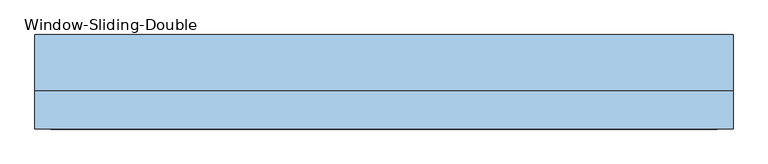
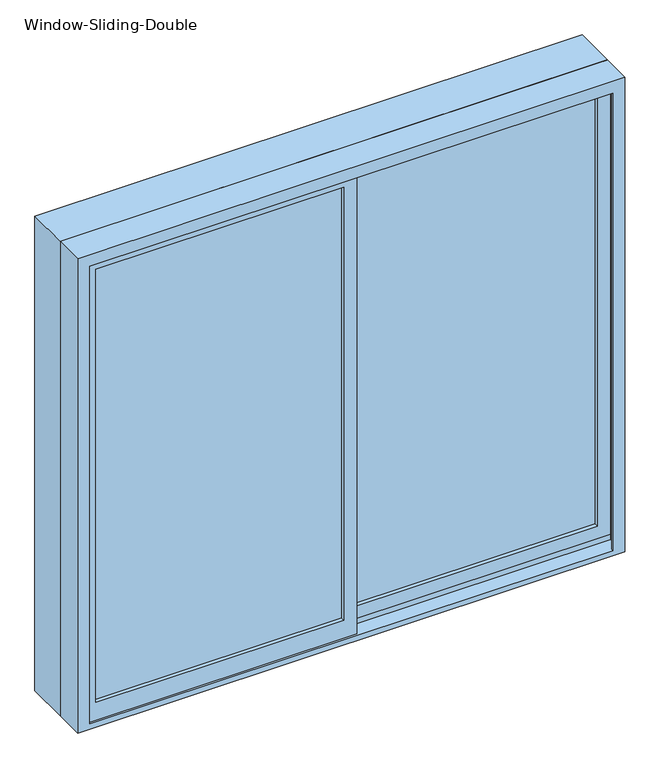
"""IFC4 building model written with IfcOpenShell, lengths in millimetres: window geometry, Window-Sliding-Double."""

from ifc_helpers import new_model, si_unit, frame, origin, place, context, project, spatial, polyline, outline, extrude, faceted_brep, source, transform, mapped, element, save


def window_sliding_double_c634d93e(model_context):
    return source(origin(), model_context, "Body", "SolidModel", [
        extrude(outline(polyline([(952.5, -22.225), (952.5, 895.35), (2571.75, 895.35), (2571.75, -22.225), (952.5, -22.225)]), holes=[polyline([(996.95, 850.9), (996.95, 22.225), (2527.3, 22.225), (2527.3, 850.9), (996.95, 850.9)])]), frame((0.0, -78.74, 0.0), z_axis=(0.0, 1.0, 0.0), x_axis=(0.0, 0.0, 1.0)), (0.0, 0.0, 1.0), 44.45),
        extrude(outline(polyline([(933.45, 22.225), (2571.75, 22.225), (2571.75, -895.35), (933.45, -895.35), (933.45, 22.225)]), holes=[polyline([(2527.3, -850.9), (2527.3, -22.225), (996.95, -22.225), (996.95, -850.9), (2527.3, -850.9)])]), frame((0.0, -123.19, 0.0), z_axis=(0.0, 1.0, 0.0), x_axis=(0.0, 0.0, 1.0)), (0.0, 0.0, 1.0), 44.45),
        extrude(outline(polyline([(-22.225, -110.49), (-850.9, -110.49), (-850.9, -104.14), (-22.225, -104.14), (-22.225, -110.49)])), frame((0.0, 0.0, 996.95), z_axis=(0.0, 0.0, 1.0), x_axis=(1.0, 0.0, 0.0)), (0.0, 0.0, 1.0), 1530.35),
        extrude(outline(polyline([(-22.225, -97.79), (-850.9, -97.79), (-850.9, -91.44), (-22.225, -91.44), (-22.225, -97.79)])), frame((0.0, 0.0, 996.95), z_axis=(0.0, 0.0, 1.0), x_axis=(1.0, 0.0, 0.0)), (0.0, 0.0, 1.0), 1530.35),
        extrude(outline(polyline([(850.9, -66.04), (22.225, -66.04), (22.225, -59.69), (850.9, -59.69), (850.9, -66.04)])), frame((0.0, 0.0, 996.95), z_axis=(0.0, 0.0, 1.0), x_axis=(1.0, 0.0, 0.0)), (0.0, 0.0, 1.0), 1530.35),
        extrude(outline(polyline([(850.9, -53.34), (22.225, -53.34), (22.225, -46.99), (850.9, -46.99), (850.9, -53.34)])), frame((0.0, 0.0, 996.95), z_axis=(0.0, 0.0, 1.0), x_axis=(1.0, 0.0, 0.0)), (0.0, 0.0, 1.0), 1530.35),
        extrude(outline(polyline([(2590.8, 914.4), (2590.8, -914.4), (914.4, -914.4), (914.4, 914.4), (2590.8, 914.4)]), holes=[polyline([(2571.75, -895.35), (2571.75, 895.35), (933.45, 895.35), (933.45, -895.35), (2571.75, -895.35)])]), frame((0.0, -27.94, 0.0), z_axis=(0.0, 1.0, 0.0), x_axis=(0.0, 0.0, 1.0)), (0.0, 0.0, 1.0), 146.05),
        faceted_brep([(-914.4, -27.94, 914.4), (914.4, -27.94, 914.4), (914.4, -129.54, 914.4), (-914.4, -129.54, 914.4), (-873.4778905, -129.54, 2549.8778905), (-873.4778905, -129.54, 933.45), (-873.4778905, -123.19, 933.45), (-873.4778905, -123.19, 2549.8778905), (-895.35, -123.19, 933.45), (-895.35, -123.19, 2571.75), (895.35, -123.19, 2571.75), (895.35, -123.19, 933.45), (873.4778905, -123.19, 933.45), (873.4778905, -123.19, 2549.8778905), (-895.35, -78.74, 933.45), (-895.35, -78.74, 952.5), (-895.35, -34.29, 952.5), (-895.35, -34.29, 933.45), (-895.35, -27.94, 933.45), (-895.35, -27.94, 2571.75), (-914.4, -27.94, 2590.8), (914.4, -27.94, 2590.8), (895.35, -27.94, 2571.75), (895.35, -27.94, 933.45), (-914.4, -129.54, 2590.8), (914.4, -129.54, 2590.8), (873.4778905, -129.54, 2549.8778905), (873.4778905, -129.54, 933.45), (895.35, -34.29, 933.45), (895.35, -34.29, 952.5), (895.35, -78.74, 952.5), (895.35, -78.74, 933.45)], [[[0, 1, 2, 3]], [[4, 5, 6, 7]], [[7, 6, 8, 9, 10, 11, 12, 13]], [[9, 8, 14, 15, 16, 17, 18, 19]], [[0, 20, 21, 1], [22, 19, 18, 23]], [[24, 20, 0, 3]], [[2, 25, 24, 3], [4, 26, 27, 5]], [[7, 13, 26, 4]], [[9, 19, 22, 10]], [[20, 24, 25, 21]], [[13, 12, 27, 26]], [[22, 23, 28, 29, 30, 31, 11, 10]], [[21, 25, 2, 1]], [[27, 12, 11, 31, 14, 8, 6, 5]], [[31, 30, 15, 14]], [[30, 29, 16, 15]], [[29, 28, 17, 16]], [[18, 17, 28, 23]]]),
    ])


if __name__ == "__main__":
    model = new_model("IFC4")
    model_context = context("Model", 3, world=origin())
    ifc_project = project(units=[si_unit("LENGTHUNIT", "METRE", prefix="MILLI")], contexts=[model_context])
    site = spatial("IfcSite", under=ifc_project)
    building = spatial("IfcBuilding", under=site)
    placement = place(None, origin())
    window_sliding_double_shape = window_sliding_double_c634d93e(model_context)
    element("IfcWindow", 1, ObjectType="Window-Sliding-Double", at=placement, inside=building, context=model_context, shape_type="MappedRepresentation", body=[
        mapped(window_sliding_double_shape, transform((0.0, 0.0, 0.0), x_axis=(1.0, 0.0, 0.0), y_axis=(0.0, 1.0, 0.0), z_axis=(0.0, 0.0, 1.0))),
    ])
    save(model, "model.ifc")

# Revit data of these elements
# Type "Window-Sliding-Double"
#   Type Mark = "19"
#   Fire Rating = "0.5h"
#   Assembly Code = "B2020100"
#   Analytic Construction = "Double glazing - domestic"
#   Window Inset [instance default] = 0' - 0"
#   Wall Thickness [instance default] = 0' - 6"
#   Visual Light Transmittance = 0.81
#   Thermal Resistance (R) = 1.8146 (h·ft²·°F)/BTU
#   Solar Heat Gain Coefficient = 0.76
#   Muntin Width = 2' - 8 5/8"
#   Muntin Height = 5' - 0 1/4"
#   Interior Wall Closure [instance default] = 0' - 2 3/4"
#   Heat Transfer Coefficient (U) = 0.5511 BTU/(h·ft²·°F)
#   Frame Extension [instance default] = 0' - 0 1/4"
#   Exterior Wall Closure [instance default] = 0' - 1 1/4"
#   Rough Width = 6' - 0 1/2"
#   Rough Height = 5' - 6 1/2"
#   Height = 5' - 6"
#   Extension Jamb [instance default] = 0' - 2 3/4"
#   Default Sill Height = 3' - 0"
#   Width = 6' - 0"
#   Interior Trim Visibility [instance default] = yes
#   Indicator Visibility [instance default] = yes
#   Exterior Trim Visibility [instance default] = yes
#   Muntin Visibility = yes
#   Extension Jamb Visibility [instance default] = yes
#   Muntin Pattern = Muntin Pattern_2x2 : Muntin Pattern_2x2
#   Interior Trim Material = Wood - Stained
#   Interior Trim = Trim-Window-Interior-Flat : Picture Frame
#   Interior Frame Material = Wood - Stained
#   Glass Panel Material = Glass
#   Exterior Trim Material = Clad - White
#   Exterior Trim = Trim-Window-Exterior-Flat : with Sill
#   Exterior Frame Material = Clad - White
#   Wall Closure = (empty or 0)
# Element 1 (IfcWindow, "Window-Sliding-Double")
#   Wall Thickness = 0' - 9"
#   Extension Jamb = 0' - 5 3/4"
#   Materials on its faces: "Wood - Stained", "Glass", "Clad - White"
# Materials
#   "Wood - Stained": class "Wood", colour RGB 224 178 126, transparency 0, Cost = 0
#   "Glass": class "Glass", colour RGB 0 128 192, transparency 0.75, Description = "Soda Lime Glass", Cost = 0
#   "Clad - White": class "Wood", colour RGB 242 242 238, transparency 0, Cost = 0
